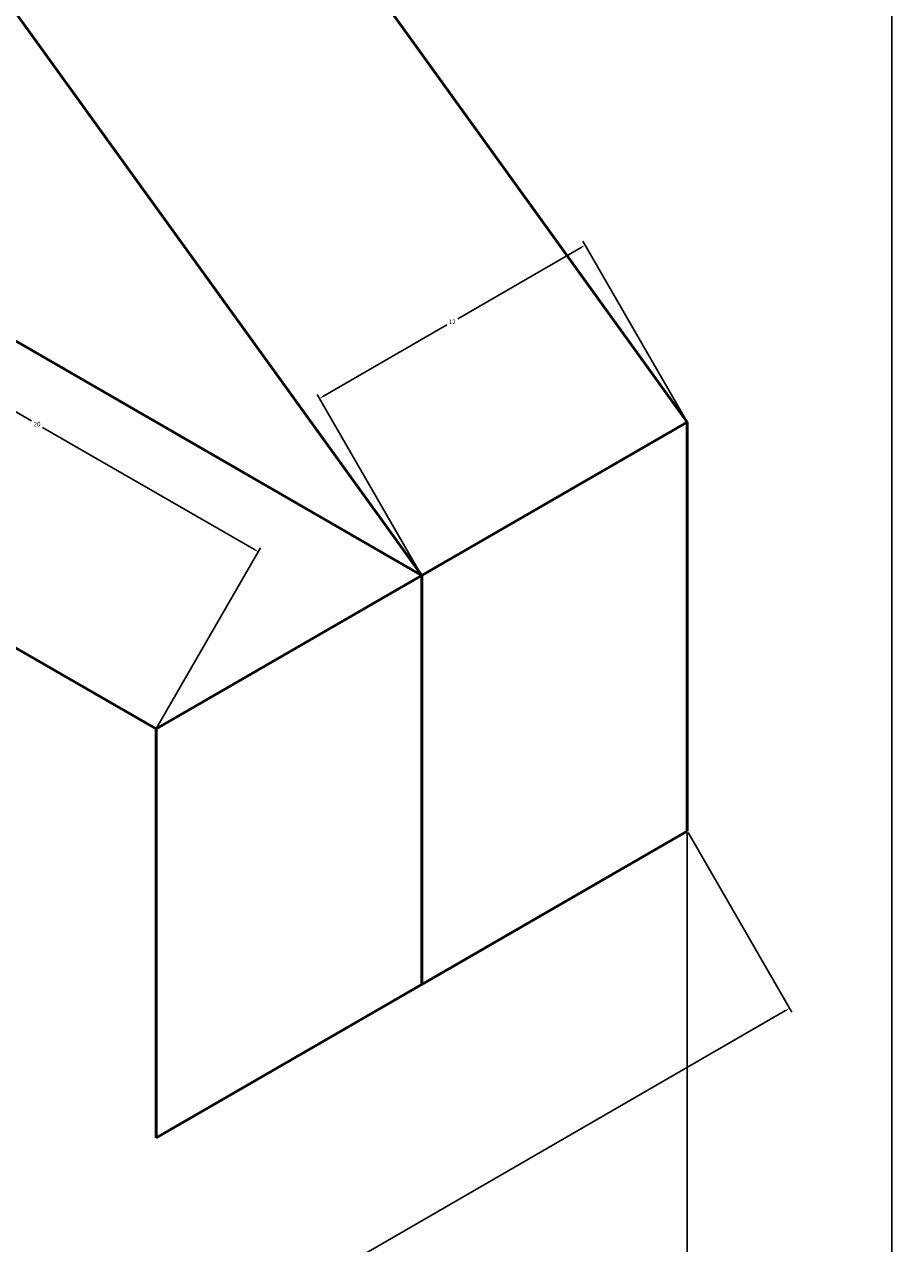
# Model space of a CAD drawing. Units: millimetres. Extents: x 2919 to 3075, y 2801 to 2951.
# Tile 13 of 14: x 3040 to 3075, y 2825 to 2872. Entities that reach past the tile are written whole.
import ezdxf

# ---------------------------------------------------------------- set-up
doc = ezdxf.new("R2010")
doc.units = ezdxf.units.MM
doc.layers.add('M-DIMS', color=2, linetype='Continuous', lineweight=18)
doc.layers.add('M-OUTL', color=7, linetype='Continuous', lineweight=50)
doc.styles.get("Standard").update_dxf_attribs({"font": 'arial.ttf'})
doc.dimstyles.get("Standard").update_dxf_attribs({"dimtxt": 0.18, "dimasz": 0.18, "dimexe": 0.18, "dimexo": 0.0625, "dimgap": 0.09, "dimtad": 0, "dimtih": 1, "dimtoh": 1, "dimdec": 4, "dimzin": 0, "dimdsep": 46, "dimtxsty": 'Standard', "dimcen": 0.09, "dimadec": 0, "dimazin": 0, "dimtfac": 1, "dimtdec": 4, "dimtofl": 0, "dimtmove": 0, "dimatfit": 3, "dimfxl": 1, "dimtolj": 1, "dimtzin": 0, "dimarcsym": 0})

# ---------------------------------------------------------------- blocks, each defined once
blk = doc.blocks.new('*D1')
at = {"layer": 'Defpoints', "color": 0, "transparency": 16777216}
for p in [(2987.323, 2944.203), (3074.337, 2944.203), (3010.912, 2808.893)]:
    blk.add_point(p, dxfattribs=at)
at = {"layer": 'M-DIMS', "color": 0, "lineweight": -2, "transparency": 16777216}
for p, q in [((2987.386, 2944.203), (3074.517, 2944.203)), ((3074.337, 2944.023), (3074.337, 2876.73)), ((3074.337, 2809.073), (3074.337, 2876.366)), ((3010.974, 2808.893), (3074.517, 2808.893))]:
    blk.add_line(p, q, dxfattribs=at)
at = {"layer": 'M-DIMS', "color": 0, "transparency": 16777216}
for points in [[(3074.307, 2944.023), (3074.367, 2944.023), (3074.337, 2944.203)], [(3074.307, 2809.073), (3074.367, 2809.073), (3074.337, 2808.893)]]:
    blk.add_solid(points, dxfattribs=at)
at = {"layer": 'M-DIMS', "color": 0, "transparency": 16777216, "insert": (3074.337, 2876.548), "char_height": 0.18, "attachment_point": 5}
blk.add_mtext('\\A1;135.3', dxfattribs=at)
blk = doc.blocks.new('*D2')
at = {"layer": 'Defpoints', "color": 0, "transparency": 16777216}
for p in [(2927.773, 2856.893), (3066.337, 2840.893), (3066.337, 2800.893)]:
    blk.add_point(p, dxfattribs=at)
at = {"layer": 'M-DIMS', "color": 0, "lineweight": -2, "transparency": 16777216}
for p, q in [((2927.773, 2856.831), (2927.773, 2800.713)), ((3066.337, 2840.831), (3066.337, 2800.713)), ((2927.953, 2800.893), (2996.6, 2800.893)), ((3066.157, 2800.893), (2997.51, 2800.893))]:
    blk.add_line(p, q, dxfattribs=at)
at = {"layer": 'M-DIMS', "color": 0, "transparency": 16777216}
for points in [[(2927.953, 2800.923), (2927.953, 2800.863), (2927.773, 2800.893)], [(3066.157, 2800.923), (3066.157, 2800.863), (3066.337, 2800.893)]]:
    blk.add_solid(points, dxfattribs=at)
at = {"layer": 'M-DIMS', "color": 0, "transparency": 16777216, "insert": (2997.055, 2800.893), "char_height": 0.18, "attachment_point": 5}
blk.add_mtext('\\A1;138.56', dxfattribs=at)
blk = doc.blocks.new('*D4')
at = {"layer": 'Defpoints', "color": 0, "transparency": 16777216}
for p in [(3066.337, 2840.893), (3010.912, 2808.893), (3014.912, 2801.965)]:
    blk.add_point(p, dxfattribs=at)
at = {"layer": 'M-DIMS', "color": 0, "lineweight": -2, "transparency": 16777216}
for p, q in [((3066.368, 2840.839), (3070.427, 2833.809)), ((3070.181, 2833.875), (3042.843, 2818.092)), ((3015.068, 2802.055), (3042.405, 2817.839)), ((3010.943, 2808.839), (3015.002, 2801.809))]:
    blk.add_line(p, q, dxfattribs=at)
at = {"layer": 'M-DIMS', "color": 0, "transparency": 16777216}
for points in [[(3070.166, 2833.901), (3070.196, 2833.849), (3070.337, 2833.965)], [(3015.053, 2802.081), (3015.083, 2802.029), (3014.912, 2801.965)]]:
    blk.add_solid(points, dxfattribs=at)
at = {"layer": 'M-DIMS', "color": 0, "transparency": 16777216, "insert": (3042.624, 2817.965), "char_height": 0.18, "attachment_point": 5}
blk.add_mtext('\\A1;64', dxfattribs=at)
blk = doc.blocks.new('*D7')
at = {"layer": 'Defpoints', "color": 0, "transparency": 16777216}
for p in [(3028.232, 2854.893), (3049.552, 2851.822), (3045.553, 2844.893)]:
    blk.add_point(p, dxfattribs=at)
at = {"layer": 'M-DIMS', "color": 0, "lineweight": -2, "transparency": 16777216}
for p, q in [((3028.263, 2854.947), (3032.321, 2861.977)), ((3032.387, 2861.731), (3040.672, 2856.948)), ((3049.397, 2851.912), (3041.112, 2856.694)), ((3045.584, 2844.947), (3049.642, 2851.977))]:
    blk.add_line(p, q, dxfattribs=at)
at = {"layer": 'M-DIMS', "color": 0, "transparency": 16777216}
for points in [[(3032.402, 2861.757), (3032.372, 2861.705), (3032.231, 2861.821)], [(3049.412, 2851.938), (3049.382, 2851.886), (3049.552, 2851.822)]]:
    blk.add_solid(points, dxfattribs=at)
at = {"layer": 'M-DIMS', "color": 0, "transparency": 16777216, "insert": (3040.892, 2856.821), "char_height": 0.18, "attachment_point": 5}
blk.add_mtext('\\A1;20', dxfattribs=at)
blk = doc.blocks.new('*D9')
at = {"layer": 'Defpoints', "color": 0, "transparency": 16777216}
for p in [(3062.337, 2863.821), (3066.337, 2856.893), (3055.945, 2850.893)]:
    blk.add_point(p, dxfattribs=at)
at = {"layer": 'M-DIMS', "color": 0, "lineweight": -2, "transparency": 16777216}
for p, q in [((3066.306, 2856.947), (3062.247, 2863.977)), ((3062.181, 2863.731), (3057.351, 2860.942)), ((3052.101, 2857.911), (3056.932, 2860.7)), ((3055.914, 2850.947), (3051.855, 2857.977))]:
    blk.add_line(p, q, dxfattribs=at)
at = {"layer": 'M-DIMS', "color": 0, "transparency": 16777216}
for points in [[(3062.166, 2863.757), (3062.196, 2863.705), (3062.337, 2863.821)], [(3052.086, 2857.937), (3052.116, 2857.885), (3051.945, 2857.821)]]:
    blk.add_solid(points, dxfattribs=at)
at = {"layer": 'M-DIMS', "color": 0, "transparency": 16777216, "insert": (3057.141, 2860.821), "char_height": 0.18, "attachment_point": 5}
blk.add_mtext('\\A1;12', dxfattribs=at)

msp = doc.modelspace()

# ---------------------------------------------------------------- linework, layer by layer
at = {"layer": 'M-OUTL'}
for p, q in [((3031.6962, 2904.8932), (3066.3372, 2856.8932)), ((3055.9449, 2850.8932), (3021.3039, 2898.8932)), ((3055.9449, 2850.8932), (3021.3039, 2870.8932)), ((3066.3372, 2856.8932), (3045.5526, 2844.8932)), ((3066.3372, 2840.8932), (3066.3372, 2856.8932)), ((3045.5526, 2844.8932), (3028.2321, 2854.8932)), ((3055.9449, 2834.8932), (3055.9449, 2850.8932)), ((3045.5526, 2828.8932), (3045.5526, 2844.8932)), ((3045.5526, 2828.8932), (3066.3372, 2840.8932)), ((3066.3372, 2840.8932), (3055.9449, 2834.8932))]:
    msp.add_line(p, q, dxfattribs=at)

# ---------------------------------------------------------------- dimensions: what is measured, and where the dimension line sits
at = {"layer": 'M-DIMS'}
for base, p1, p2, angle, override, picture, middle in [((3074.3372, 2944.2026), (3010.9116, 2808.8932), (2987.3232, 2944.2026), 90, {"dimdec": 1, "dimlfac": 1, "dimrnd": 0, "dimzin": 0, "dimdsep": 46, "dimlunit": 2}, '*D1', (3074.3372, 2876.5479)), ((3062.3372, 2863.8214), (3055.9449, 2850.8932), (3066.3372, 2856.8932), 30, {"dimdec": 0, "dimlfac": 1, "dimrnd": 0, "dimzin": 0, "dimdsep": 46, "dimlunit": 2}, '*D9', (3057.1411, 2860.8214)), ((3049.5525, 2851.8216), (3028.2316, 2854.8929), (3045.5526, 2844.8932), 330.00155, {"dimdec": 0, "dimlfac": 1, "dimrnd": 0, "dimzin": 0, "dimdsep": 46, "dimlunit": 2}, '*D7', (3040.8919, 2856.8214)), ((3014.9116, 2801.965), (3066.3372, 2840.8932), (3010.9116, 2808.8932), 210, {"dimdec": 0, "dimlfac": 1, "dimrnd": 0, "dimzin": 0, "dimdsep": 46, "dimlunit": 2}, '*D4', (3042.6244, 2817.965))]:
    dim = msp.add_linear_dim(base=base, p1=p1, p2=p2, angle=angle, dimstyle='Standard', override=override, dxfattribs=at)
    dim.commit()
    dim.dimension.update_dxf_attribs({"geometry": picture, "text_midpoint": middle})
dim = msp.add_linear_dim(base=(3066.3372, 2800.8932), p1=(2927.7732, 2856.8932), p2=(3066.3372, 2840.8932), dimstyle='Standard', override={"dimdec": 2, "dimlfac": 1, "dimrnd": 0, "dimzin": 0, "dimdsep": 46, "dimlunit": 2}, dxfattribs=at)
dim.commit()
dim.dimension.update_dxf_attribs({"geometry": '*D2', "text_midpoint": (2997.0552, 2800.8932)})

doc.saveas('drawing.dxf')
